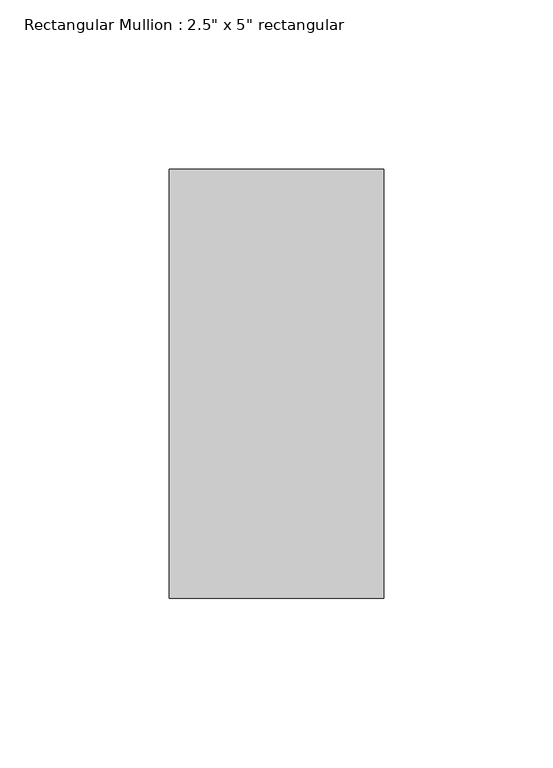
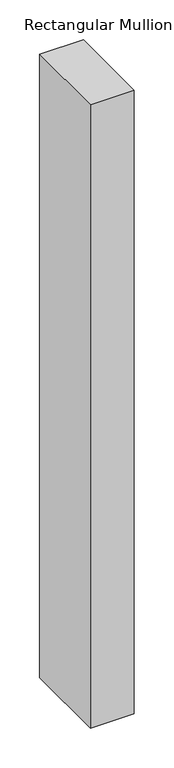
"""IFC4 building model written with IfcOpenShell, lengths in millimetres: member geometry."""

from ifc_helpers import new_model, si_unit, frame, origin, place, context, project, spatial, polyline, outline, extrude, source, transform, mapped, element, save


def member_e49f56fc(model_context):
    return source(origin(), model_context, "Body", "SweptSolid", [
        extrude(outline(polyline([(31.75, 63.5), (31.75, -63.5), (-31.75, -63.5), (-31.75, 63.5), (31.75, 63.5)])), frame((0.0, 0.0, -954.0158113), z_axis=(0.0, 0.0, 1.0), x_axis=(1.0, 0.0, 0.0)), (0.0, 0.0, 1.0), 954.0158113),
    ])


if __name__ == "__main__":
    model = new_model("IFC4")
    model_context = context("Model", 3, world=origin())
    ifc_project = project(units=[si_unit("LENGTHUNIT", "METRE", prefix="MILLI")], contexts=[model_context])
    site = spatial("IfcSite", under=ifc_project)
    building = spatial("IfcBuilding", under=site)
    placement = place(None, origin())
    member_shape = member_e49f56fc(model_context)
    element("IfcMember", 1, ObjectType="Rectangular Mullion : 2.5\" x 5\" rectangular", at=placement, inside=building, context=model_context, shape_type="MappedRepresentation", body=[
        mapped(member_shape, transform((0.0, 0.0, 0.0), x_axis=(1.0, 0.0, 0.0), y_axis=(0.0, 1.0, 0.0), z_axis=(0.0, 0.0, 1.0))),
    ])
    save(model, "model.ifc")

# Revit data of these elements
# Type "Rectangular Mullion : 2.5\" x 5\" rectangular"
#   built-in parameter 1007304 = 0.416667 (stored number, unit not read)
#   built-in parameter 1007301 = 0.104167 (stored number, unit not read)
#   built-in parameter 1007300 = 0.104167 (stored number, unit not read)
# Element 1 (IfcMember, "Rectangular Mullion : 2.5\" x 5\" rectangular")
#   Materials on its faces: "Aluminum"
# Materials
#   "Aluminum": class "Metal", colour RGB 247 247 247, transparency 0, Description = "Aluminum 6061", Cost = 0
